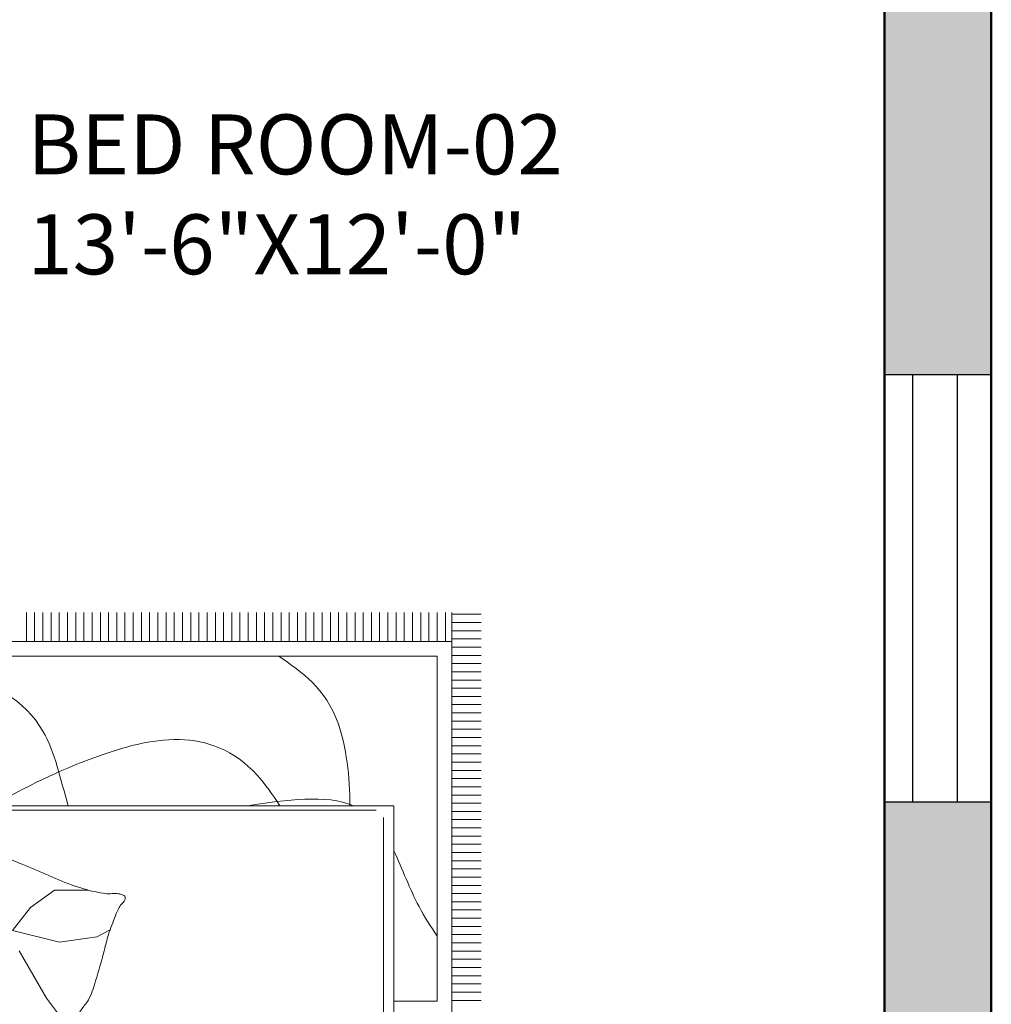
# Model space of a CAD drawing. Units: inches. Extents: x -7 to 1228, y -146 to 1091.
# Tile 39 of 88: x 1045 to 1127, y 117 to 200. Entities that reach past the tile are written whole.
import ezdxf

# ---------------------------------------------------------------- set-up
doc = ezdxf.new("R2010")
doc.units = ezdxf.units.IN
for name, color, linetype, lineweight in [('A-AREA-IDEN', 7, 'Continuous', 18), ('A-FURN', 8, 'Continuous', 18), ('A-GLAZ', 175, 'Continuous', 25), ('A-WALL', 7, 'Continuous', 50), ('A-WALL-PATT', 251, 'Continuous', 13)]:
    doc.layers.add(name, color=color, linetype=linetype, lineweight=lineweight)
doc.styles.add('DIM_FONT', font='SIMPLEX.shx', dxfattribs={"width": 0.8})
doc.styles.get("Standard").update_dxf_attribs({"font": 'arial.ttf'})

# ---------------------------------------------------------------- blocks, each defined once
blk = doc.blocks.new('A$C4F634EDD')
for p, q in [((2.3, 2.6295), (2.3, 0.5295)), ((2.2716, 0.5617), (2.2716, 1.7136)), ((1.4276, 1.1611), (1.3484, 1.0571)), ((2.4588, 1.1852), (2.4588, 0)), ((1.3484, 1.0571), (1.2733, 0.9268)), ((2.3, 1.0652), (2.4188, 1.0652)), ((2.4188, 1.0652), (2.4188, 0.12)), ((2.4588, 1.0628), (2.5388, 1.0628)), ((2.4588, 1.0403), (2.5388, 1.0403)), ((2.4588, 1.0178), (2.5388, 1.0178)), ((2.4588, 0.9953), (2.5388, 0.9953)), ((2.4588, 0.9728), (2.5388, 0.9728)), ((2.4588, 0.9503), (2.5388, 0.9503)), ((2.4588, 0.9278), (2.5388, 0.9278)), ((1.2555, 0.8715), (1.384, 0.9031)), ((1.384, 0.9031), (1.4868, 0.8892)), ((2.4588, 0.9053), (2.5388, 0.9053)), ((1.2555, 0.8715), (1.3049, 0.8082)), ((1.4868, 0.8892), (1.5228, 0.8692)), ((2.4588, 0.8828), (2.5388, 0.8828)), ((2.4588, 0.8603), (2.5388, 0.8603)), ((2.4588, 0.8378), (2.5388, 0.8378)), ((2.4588, 0.8153), (2.5388, 0.8153)), ((1.3049, 0.8082), (1.3701, 0.7608)), ((2.4588, 0.7928), (2.5388, 0.7928)), ((1.3701, 0.7608), (1.463, 0.7608)), ((2.4588, 0.7703), (2.5388, 0.7703)), ((2.4588, 0.7478), (2.5388, 0.7478)), ((2.4588, 0.7253), (2.5388, 0.7253)), ((2.4588, 0.7028), (2.5388, 0.7028)), ((2.4588, 0.6803), (2.5388, 0.6803)), ((2.4588, 0.6578), (2.5388, 0.6578)), ((2.4588, 0.6353), (2.5388, 0.6353)), ((2.4588, 0.6128), (2.5388, 0.6128)), ((2.4588, 0.5903), (2.5388, 0.5903)), ((2.4588, 0.5678), (2.5388, 0.5678)), ((0.5458, 0.5417), (2.2516, 0.5417)), ((2.4588, 0.5453), (2.5388, 0.5453)), ((2.3, 0.5295), (0.5, 0.5295)), ((2.4588, 0.5228), (2.5388, 0.5228)), ((2.4588, 0.5003), (2.5388, 0.5003)), ((2.4588, 0.4778), (2.5388, 0.4778)), ((2.4588, 0.4553), (2.5388, 0.4553)), ((2.4588, 0.4328), (2.5388, 0.4328)), ((2.4588, 0.4103), (2.5388, 0.4103)), ((2.4588, 0.3878), (2.5388, 0.3878)), ((2.4588, 0.3653), (2.5388, 0.3653)), ((2.4588, 0.3428), (2.5388, 0.3428)), ((2.4588, 0.3203), (2.5388, 0.3203)), ((2.4588, 0.2978), (2.5388, 0.2978)), ((2.4588, 0.2753), (2.5388, 0.2753)), ((2.4588, 0.2528), (2.5388, 0.2528)), ((2.4588, 0.2303), (2.5388, 0.2303)), ((2.4588, 0.2078), (2.5388, 0.2078)), ((2.4588, 0.1853), (2.5388, 0.1853)), ((2.4588, 0.1628), (2.5388, 0.1628)), ((2.4588, 0.1403), (2.5388, 0.1403)), ((2.4188, 0.12), (0.3786, 0.12)), ((2.4588, 0.1178), (2.5388, 0.1178)), ((2.4588, 0.0953), (2.5388, 0.0953)), ((2.4588, 0.08), (0.3386, 0.08)), ((1.2936, 0), (1.2936, 0.08)), ((1.3161, 0), (1.3161, 0.08)), ((1.3386, 0), (1.3386, 0.08)), ((1.3611, 0), (1.3611, 0.08)), ((1.3836, 0), (1.3836, 0.08)), ((1.4061, 0), (1.4061, 0.08)), ((1.4286, 0), (1.4286, 0.08)), ((1.4511, 0), (1.4511, 0.08)), ((1.4736, 0), (1.4736, 0.08)), ((1.4961, 0), (1.4961, 0.08)), ((1.5186, 0), (1.5186, 0.08)), ((1.5411, 0), (1.5411, 0.08)), ((1.5636, 0), (1.5636, 0.08)), ((1.5861, 0), (1.5861, 0.08)), ((1.6086, 0), (1.6086, 0.08)), ((1.6311, 0), (1.6311, 0.08)), ((1.6536, 0), (1.6536, 0.08)), ((1.6761, 0), (1.6761, 0.08)), ((1.6986, 0), (1.6986, 0.08)), ((1.7211, 0), (1.7211, 0.08)), ((1.7436, 0), (1.7436, 0.08)), ((1.7661, 0), (1.7661, 0.08)), ((1.7886, 0), (1.7886, 0.08)), ((1.8111, 0), (1.8111, 0.08)), ((1.8336, 0), (1.8336, 0.08)), ((1.8561, 0), (1.8561, 0.08)), ((1.8786, 0), (1.8786, 0.08)), ((1.9011, 0), (1.9011, 0.08)), ((1.9236, 0), (1.9236, 0.08)), ((1.9461, 0), (1.9461, 0.08)), ((1.9686, 0), (1.9686, 0.08)), ((1.9911, 0), (1.9911, 0.08)), ((2.0136, 0), (2.0136, 0.08)), ((2.0361, 0), (2.0361, 0.08)), ((2.0586, 0), (2.0586, 0.08)), ((2.0811, 0), (2.0811, 0.08)), ((2.1036, 0), (2.1036, 0.08)), ((2.1261, 0), (2.1261, 0.08)), ((2.1486, 0), (2.1486, 0.08)), ((2.1711, 0), (2.1711, 0.08)), ((2.1936, 0), (2.1936, 0.08)), ((2.2161, 0), (2.2161, 0.08)), ((2.2386, 0), (2.2386, 0.08)), ((2.2611, 0), (2.2611, 0.08)), ((2.2836, 0), (2.2836, 0.08)), ((2.3061, 0), (2.3061, 0.08)), ((2.3286, 0), (2.3286, 0.08)), ((2.3511, 0), (2.3511, 0.08)), ((2.3736, 0), (2.3736, 0.08)), ((2.3961, 0), (2.3961, 0.08)), ((2.4186, 0), (2.4186, 0.08)), ((2.4411, 0), (2.4411, 0.08)), ((2.4588, 0.0728), (2.5388, 0.0728)), ((2.4588, 0.0503), (2.5388, 0.0503)), ((2.4588, 0.0278), (2.5388, 0.0278)), ((2.4588, 0.0053), (2.5388, 0.0053))]:
    blk.add_line(p, q)
for centre, radius, start, end in [((1.6045, 1.1973), 0.194, 210.9056, 219.7005), ((1.3929, 1.0217), 0.081, 26.0735, 39.7005), ((1.2892, 0.9709), 0.1965, 17.8396, 26.0735), ((-0.4304, 0.4175), 2.003, 15.2625, 17.8396), ((-0.0881, 0.5109), 1.6481, 13.841, 15.2625), ((2.0418, 1.0357), 0.5454, 193.841, 196.3122), ((1.6908, 0.933), 0.1798, 196.3122, 200.7773), ((4.0115, 1.8135), 2.6619, 200.7773, 201.9373), ((1.6124, 0.8472), 0.0755, 201.9373, 225.0955), ((1.5473, 0.7819), 0.0168, 354.6428, 45.0955), ((1.6266, 0.159), 0.6236, 106.3527, 113.0962), ((1.5721, 0.3449), 0.43, 98.2293, 106.3527), ((1.5195, 0.708), 0.063, 82.216, 98.2293), ((1.5362, 0.8298), 0.0599, 262.216, 278.6443), ((1.5375, 0.8209), 0.0509, 278.6443, 297.2959), ((1.5582, 0.7808), 0.0058, 297.2959, 354.6428), ((3.6722, -4.6377), 5.8383, 113.0962, 113.45234), ((0.5234, 2.5582), 2.0162, 292.0188, 293.104), ((-1.0798, 6.3161), 6.1019, 293.10398, 293.45234), ((2.4404, -2.1823), 3.0972, 112.0188, 112.8944)]:
    blk.add_arc(centre, radius, start, end)
for points, knots in [([(2.3, 0.6535), (2.3236, 0.7026), (2.3554, 0.7914), (2.4015, 0.8608), (2.4188, 0.8868)], [1893.525221, 1893.525221, 1893.525221, 1893.525221, 2051.902476, 2146.74457, 2146.74457, 2146.74457, 2146.74457]), ([(0.7187, 0.12), (0.9791, 0.1362), (1.326, 0.1577), (1.3868, 0.4574), (1.408, 0.5295)], [0, 0, 0, 0, 653.160442, 870.050857, 870.050857, 870.050857, 870.050857]), ([(1.2016, 0.5295), (1.2892, 0.479), (1.5144, 0.3684), (1.8265, 0.2994), (1.9681, 0.4992), (1.9875, 0.5295)], [936.534237, 936.534237, 936.534237, 936.534237, 1243.285375, 1683.261222, 1758.254386, 1758.254386, 1758.254386, 1758.254386]), ([(2.1796, 0.5295), (2.1798, 0.4519), (2.1548, 0.2369), (2.0487, 0.164), (1.9846, 0.12)], [2202.034493, 2202.034493, 2202.034493, 2202.034493, 2357.807635, 2594.446174, 2594.446174, 2594.446174, 2594.446174])]:
    blk.add_open_spline(points, degree=3, knots=knots)
blk.add_open_spline([(1.9003, 0.5295), (2.0065, 0.514), (2.1132, 0.4978), (2.1894, 0.5295)], degree=3)
at = {"style": 'DIM_FONT', "width": 0.8, "flags": 9}
for tag, p in [('YSIZE', (0.5, 2.6295)), ('XSIZE', (0.5, 2.6295)), ('XSIZE', (2.2985, 2.6295)), ('YSIZE', (2.2985, 2.6295))]:
    blk.add_attdef(tag, p, '', height=0.0005, dxfattribs=at)
blk = doc.blocks.new('WIN-36')
for p, q in [((0, 36), (0, 0)), ((9, 36), (0, 36)), ((2.343, 36), (2.343, 0)), ((6.137, 0), (6.137, 36)), ((9, 0), (9, 36)), ((0, 0), (9, 0)), ((2.343, 0), (6.137, 0))]:
    blk.add_line(p, q)

msp = doc.modelspace()

# ---------------------------------------------------------------- hatches: boundary and pattern name
at = {"layer": 'A-WALL-PATT'}
h = msp.add_hatch(color=256, dxfattribs=at)
h.dxf.hatch_style = 1
h.paths.add_polyline_path([(69, 568), (60, 568), (60, 493), (63.289, 493), (69, 493)])
h.paths.add_polyline_path([(69, 662.405), (60, 662.405), (60, 586), (69, 586)], flags=17)
h.paths.add_polyline_path([(69, 723), (184, 723), (184, 734), (179, 734), (179, 728), (69, 728), (69, 741.623), (60, 741.623), (60, 698.405), (69, 698.405)], flags=17)
h.paths.add_polyline_path([(69, 782), (231, 782), (231, 728), (231, 723), (231, 586), (236, 586), (236, 787), (69, 787), (69, 800.126), (60, 800.126), (60, 765.623), (69, 765.623)])
h.paths.add_polyline_path([(184, 842), (189, 842), (189, 848), (173, 848), (173, 842), (179, 842), (179, 787), (184, 787)])
h.paths.add_polyline_path([(118.22, 69), (69, 69), (69, 60), (118.22, 60)])
h.paths.add_polyline_path([(227, 69), (154.22, 69), (154.22, 60), (227, 60)])
h.paths.add_polyline_path([(236, 60), (232.711, 60), (227, 60), (227, 36), (236, 36)])
h.paths.add_polyline_path([(389, 60), (380, 60), (380, 36), (389, 36)])
h.paths.add_polyline_path([(384, 181), (380, 181), (380, 115), (380, 78), (384, 78)])
h.paths.add_polyline_path([(380, 115), (334.547, 115), (334.547, 109), (380, 109)])
h.paths.add_polyline_path([(274.547, 115), (236, 115), (236, 201), (232.711, 201), (231, 201), (231, 78), (236, 78), (236, 109), (274.547, 109)])
h.paths.add_polyline_path([(69, 123), (60, 123), (60, 78), (69, 78)])
h.paths.add_polyline_path([(69, 201), (60, 201), (60, 159), (69, 159)])
h.paths.add_polyline_path([(143, 219), (69, 219), (69, 213), (143, 213)], flags=17)
h.paths.add_polyline_path([(189, 219), (184, 219), (184, 274), (231, 274), (231, 219), (236, 219), (236, 279), (184, 279), (184, 297), (179, 297), (179, 279), (69, 279), (69, 290.912), (60, 290.912), (60, 262.179), (69, 262.179), (69, 274), (179, 274), (179, 219), (173, 219), (173, 213), (189, 213)])
h.paths.add_polyline_path([(69, 238.179), (60, 238.179), (60, 219), (69, 219)], flags=17)
h.paths.add_polyline_path([(69, 333), (60, 333), (60, 314.912), (69, 314.912), (69, 316.965)])
h.paths.add_polyline_path([(190, 338), (184, 338), (69, 338), (69, 333), (179, 333), (179, 327), (184, 327), (184, 333.021), (190, 333.046)])
h.paths.add_polyline_path([(69, 386.806), (60, 386.806), (60, 351), (69, 351)])
h.paths.add_polyline_path([(69, 475), (60, 475), (60, 422.806), (69, 422.806)])
h.paths.add_polyline_path([(236, 475), (231, 475), (231, 351.238), (236, 351.238)])
h.paths.add_polyline_path([(384, 475), (380, 475), (380, 362), (384, 362)])
h.paths.add_polyline_path([(547, 307), (439, 307), (439, 356), (445, 356), (445, 362), (433, 362), (433, 307), (380, 307), (380, 244), (380, 241), (384, 241), (384, 301), (433, 301), (433, 277), (439, 277), (439, 301), (547, 301)])
h.paths.add_polyline_path([(547, 241), (439, 241), (439, 247), (433, 247), (433, 235), (547, 235)])
h.paths.add_polyline_path([(450, 69), (440.286, 69), (424.889, 69), (389, 69), (389, 60), (450, 60)])
h.paths.add_polyline_path([(547, 69), (486, 69), (486, 60), (547, 60)])
h.paths.add_polyline_path([(556, 148.268), (547, 148.268), (547, 78), (556, 78)])
h.paths.add_polyline_path([(556, 223), (547, 223), (547, 195), (547, 184.268), (556, 184.268)])
h.paths.add_polyline_path([(556, 311.192), (547, 311.192), (547, 273.075), (556, 273.075)])
h.paths.add_polyline_path([(556, 344), (552.711, 344), (547, 344), (547, 335.192), (556, 335.192)])
h.paths.add_polyline_path([(556, 249.075), (547, 249.075), (547, 241), (556, 241)])
h.paths.add_polyline_path([(547, 362), (475, 362), (475, 356), (547, 356)], flags=0)
h.paths.add_polyline_path([(556, 399.621), (547, 399.621), (547, 362), (556, 362)])
h.paths.add_polyline_path([(556, 475), (547, 475), (547, 435.621), (556, 435.621)])
h.paths.add_polyline_path([(547, 493), (389, 493), (389, 487), (547, 487)])
h.paths.add_polyline_path([(380, 493), (278, 493), (278, 487), (380, 487)])
h.paths.add_polyline_path([(227, 493), (69, 493), (69, 487), (227, 487)])
h.paths.add_polyline_path([(643, 122.445), (634, 122.445), (634, 78), (643, 78)])
h.paths.add_polyline_path([(702.5, 69), (692.786, 69), (677.389, 69), (643, 69), (643, 60), (702.5, 60)])
h.paths.add_polyline_path([(798, 69), (738.5, 69), (738.5, 60), (798, 60)])
h.paths.add_polyline_path([(807, 60), (803.711, 60), (798, 60), (798, 36), (807, 36)])
h.paths.add_polyline_path([(807, 109), (846.751, 109), (846.751, 115), (807, 115), (807, 159), (802, 159), (802, 78), (807, 78)])
h.paths.add_polyline_path([(807, 201), (802, 201), (802, 195), (807, 195)])
h.paths.add_polyline_path([(643, 201), (634, 201), (634, 158.445), (643, 158.445)])
h.paths.add_polyline_path([(756, 225), (751, 225), (751, 219), (643, 219), (643, 213), (756, 213)])
h.paths.add_polyline_path([(643, 240.848), (634, 240.848), (634, 219), (643, 219)])
h.paths.add_polyline_path([(643, 274), (643, 288.629), (634, 288.629), (634, 264.848), (643, 264.848)])
h.paths.add_polyline_path([(802, 279), (756, 279), (756, 297), (751, 297), (751, 279), (643, 279), (643, 274), (751, 274), (751, 255), (756, 255), (756, 274), (802, 274)])
h.paths.add_polyline_path([(807, 333), (803.711, 333), (802, 333), (802, 279), (802, 274), (802, 219), (807, 219)])
h.paths.add_polyline_path([(956, 182), (951, 182), (951, 115), (906.751, 115), (906.751, 109), (951, 109), (951, 78), (956, 78)])
h.paths.add_polyline_path([(960, 60), (951, 60), (951, 36), (960, 36)])
h.paths.add_polyline_path([(1021, 69), (1005.781, 69), (960, 69), (960, 60), (1021, 60)])
h.paths.add_polyline_path([(956, 224), (951, 224), (951, 218), (956, 218)])
h.paths.add_polyline_path([(956, 302), (1004, 302), (1004, 278), (1010, 278), (1010, 302), (1118, 302), (1118, 290.809), (1127, 290.809), (1127, 326.968), (1118, 326.968), (1118, 320.966), (1118, 307), (1010, 307), (1010, 356), (1016, 356), (1016, 362), (1004, 362), (1004, 307), (951, 307), (951, 244), (951, 242), (954.289, 242), (956, 242)])
h.paths.add_polyline_path([(643, 333), (634, 333), (634, 312.629), (643, 312.629), (643, 316.965)])
h.paths.add_polyline_path([(756, 338), (643, 338), (643, 333), (751, 333), (751, 327), (756, 327)])
h.paths.add_polyline_path([(643, 388), (634, 388), (634, 351), (643, 351)])
h.paths.add_polyline_path([(807, 357), (802, 357), (802, 351), (807, 351)])
h.paths.add_polyline_path([(807, 475), (802, 475), (802, 393), (807, 393)])
h.paths.add_polyline_path([(643, 475), (634, 475), (634, 424), (643, 424)])
h.paths.add_polyline_path([(798, 493), (643, 493), (643, 487), (798, 487)])
h.paths.add_polyline_path([(634, 493), (556, 493), (556, 487), (634, 487)])
h.paths.add_polyline_path([(813, 493), (807, 493), (807, 487), (813, 487)])
h.paths.add_polyline_path([(951, 493), (849, 493), (849, 487), (951, 487)])
h.paths.add_polyline_path([(956, 484), (951, 484), (951, 374), (956, 374)])
h.paths.add_polyline_path([(1109, 493), (969, 493), (969, 487), (1109, 487)])
h.paths.add_polyline_path([(1127, 484), (1118, 484), (1118, 450.641), (1127, 450.641)])
h.paths.add_polyline_path([(1127, 414.641), (1118, 414.641), (1118, 365), (1127, 365)])
h.paths.add_polyline_path([(1109, 362), (1046, 362), (1046, 356), (1109, 356)], flags=17)
h.paths.add_polyline_path([(1127, 356), (1123.454, 356), (1118, 356), (1118, 350.968), (1127, 350.968)], flags=0)
h.paths.add_polyline_path([(1127, 266.809), (1118, 266.809), (1118, 262.361), (1118, 242), (1127, 242)], flags=17)
h.paths.add_polyline_path([(1118, 242), (1010, 242), (1010, 248), (1004, 248), (1004, 237), (1118, 237)])
h.paths.add_polyline_path([(1127, 224), (1118, 224), (1118, 170), (1127, 170)])
h.paths.add_polyline_path([(1127, 134), (1118, 134), (1118, 78), (1127, 78)])
h.paths.add_polyline_path([(1118, 69), (1057, 69), (1057, 60), (1118, 60)])
h.paths.add_polyline_path([(227, 571.546), (227, 574), (69, 574), (69, 568), (227, 568)])
h.paths.add_polyline_path([(380, 571.546), (380, 574), (278, 574), (278, 568), (380, 568)])
h.paths.add_polyline_path([(242, 574), (236, 574), (236, 568), (242, 568)])
h.paths.add_polyline_path([(547, 571.546), (547, 574), (389, 574), (389, 568), (547, 568)])
h.paths.add_polyline_path([(384, 733), (380, 733), (380, 586), (384, 586)])
h.paths.add_polyline_path([(556, 646), (634, 646), (634, 655), (547, 655), (547, 586), (556, 586)])
h.paths.add_polyline_path([(634, 574), (556, 574), (556, 568), (634, 568)])
h.paths.add_polyline_path([(643, 655), (634, 655), (634, 586), (643, 586)])
h.paths.add_polyline_path([(798, 574), (643, 574), (643, 568), (798, 568)])
h.paths.add_polyline_path([(643, 663.854), (634, 663.854), (634, 655), (643, 655)])
h.paths.add_polyline_path([(556, 676.967), (547, 676.967), (547, 655), (556, 655)])
h.paths.add_polyline_path([(556, 733), (547, 733), (547, 712.967), (556, 712.967)])
h.paths.add_polyline_path([(643, 710), (634, 710), (634, 699.854), (643, 699.854)])
h.paths.add_polyline_path([(807, 668), (802, 668), (802, 586), (807, 586)])
h.paths.add_polyline_path([(951, 574), (849, 574), (849, 568), (951, 568)])
h.paths.add_polyline_path([(956, 691), (951, 691), (951, 577), (956, 577)])
h.paths.add_polyline_path([(1109, 574), (969, 574), (969, 568), (1109, 568)])
h.paths.add_polyline_path([(1127, 643.403), (1118, 643.403), (1118, 577), (1127, 577)])
h.paths.add_polyline_path([(1127, 568), (1123.454, 568), (1118, 568), (1118, 493), (1127, 493)])
h.paths.add_polyline_path([(1127, 733), (1118, 733), (1118, 679.403), (1127, 679.403)])
h.paths.add_polyline_path([(1127, 777.348), (1118, 777.348), (1118, 770.035), (1118, 751), (1127, 751)], flags=17)
h.paths.add_polyline_path([(1118, 751), (1010, 751), (1010, 757), (1004, 757), (1004, 745), (1118, 745)])
h.paths.add_polyline_path([(956, 811), (1004, 811), (1004, 787), (1010, 787), (1010, 811), (1017.874, 811), (1017.874, 811.627, -0.414214), (1018.247, 812), (1031.978, 812, -0.414214), (1032.351, 811.627), (1032.351, 811), (1118, 811), (1118, 801.348), (1127, 801.348), (1127, 834.685), (1118, 834.685), (1118, 830.238), (1118, 817), (1010, 817), (1010, 866), (1016, 866), (1016, 872), (1004, 872), (1004, 817), (956, 817), (956, 866), (951, 866), (951, 751), (954.289, 751), (956, 751)])
h.paths.add_polyline_path([(1118, 872), (1046, 872), (1046, 866), (1118, 866)], flags=17)
h.paths.add_polyline_path([(1127, 924.711), (1118, 924.711), (1118, 884), (1127, 884)])
h.paths.add_polyline_path([(1127, 866), (1123.711, 866), (1118, 866), (1118, 858.685), (1127, 858.685)], flags=17)
h.paths.add_polyline_path([(956, 983), (951, 983), (951, 952), (807, 952), (807, 983), (802, 983), (802, 902), (807, 902), (807, 946), (951, 946), (951, 884), (956, 884)])
h.paths.add_polyline_path([(807, 842), (802, 842), (802, 787), (756, 787), (756, 806), (751, 806), (751, 787), (643, 787), (643, 782), (751, 782), (751, 764), (756, 764), (756, 782), (802, 782), (802, 728), (807, 728)])
h.paths.add_polyline_path([(756, 848), (643, 848), (643, 842), (751, 842), (751, 836), (756, 836)])
h.paths.add_polyline_path([(756, 734), (751, 734), (751, 728), (643, 728), (643, 723), (756, 723)])
h.paths.add_polyline_path([(643, 749.791), (634, 749.791), (634, 728), (637.289, 728), (643, 728)])
h.paths.add_polyline_path([(643, 805.405), (634, 805.405), (634, 773.791), (643, 773.791)])
h.paths.add_polyline_path([(643, 896.663), (634, 896.663), (634, 860), (637.289, 860), (643, 860)])
h.paths.add_polyline_path([(643, 842), (634, 842), (634, 829.405), (643, 829.405)])
h.paths.add_polyline_path([(643, 983), (634, 983), (634, 932.663), (643, 932.663)])
h.paths.add_polyline_path([(1127, 983), (1118, 983), (1118, 960.711), (1127, 960.711)])
h.paths.add_polyline_path([(1118, 1001), (1077.525, 1001), (1077.525, 992), (1118, 992)])
h.paths.add_polyline_path([(1041.525, 1001), (960, 1001), (960, 992), (1041.525, 992)])
h.paths.add_polyline_path([(960, 1025), (951, 1025), (951, 1001), (954.289, 1001), (960, 1001)])
h.paths.add_polyline_path([(807, 1025), (798, 1025), (798, 1001), (807, 1001)])
h.paths.add_polyline_path([(798, 1001), (738.5, 1001), (738.5, 992), (798, 992)])
h.paths.add_polyline_path([(702.5, 1001), (643, 1001), (643, 992), (702.5, 992)])
h.paths.add_polyline_path([(547, 1001), (499.113, 1001), (499.113, 992), (547, 992)])
h.paths.add_polyline_path([(463.113, 1001), (389, 1001), (389, 992), (463.113, 992)])
h.paths.add_polyline_path([(389, 1025), (380, 1025), (380, 1022), (380, 1001), (383.289, 1001), (389, 1001)])
h.paths.add_polyline_path([(236, 1025), (227, 1025), (227, 1001), (236, 1001)])
h.paths.add_polyline_path([(236, 983), (231, 983), (231, 860), (236, 860)])
h.paths.add_polyline_path([(274.547, 952), (236, 952), (236, 946), (274.547, 946)])
h.paths.add_polyline_path([(380, 952), (334.547, 952), (334.547, 946), (380, 946)])
h.paths.add_polyline_path([(384, 983), (380, 983), (380, 884), (383.289, 884), (384, 884)])
h.paths.add_polyline_path([(227, 1001), (155.012, 1001), (155.012, 992), (162.875, 992), (227, 992)])
h.paths.add_polyline_path([(119.012, 1001), (69, 1001), (69, 992), (119.012, 992)])
h.paths.add_polyline_path([(69, 983), (60, 983), (60, 922.987), (69, 922.987)])
h.paths.add_polyline_path([(69, 886.987), (60, 886.987), (60, 860), (63.289, 860), (69, 860)])
h.paths.add_polyline_path([(143, 848), (69, 848), (69, 842), (143, 842)])

# ---------------------------------------------------------------- linework, layer by layer
at = {"layer": 'A-WALL'}
for p, q in [((1127, 60), (1127, 1001)), ((1118, 60), (1118, 302)), ((1118, 244), (1118, 60))]:
    msp.add_line(p, q, dxfattribs=at)

# ---------------------------------------------------------------- block references
at = {"layer": 'A-FURN', "xscale": -30.79356024027943, "yscale": 30.79356024027943, "zscale": 30.79356024027943, "rotation": 180}
msp.add_blockref('A$C4F634EDD', (1005.781, 149.972), dxfattribs=at)
at = {"layer": 'A-GLAZ'}
msp.add_blockref('WIN-36', (1118, 134), dxfattribs=at)

# ---------------------------------------------------------------- texts
at = {"layer": 'A-AREA-IDEN', "insert": (1045.691, 191.976), "char_height": 5.05676, "attachment_point": 1}
msp.add_mtext_dynamic_manual_height_columns('BED ROOM-02\\P13\'-6"X12\'-0"', width=137.28212, gutter_width=25.284, heights=[0], dxfattribs=at)

doc.saveas('drawing.dxf')
